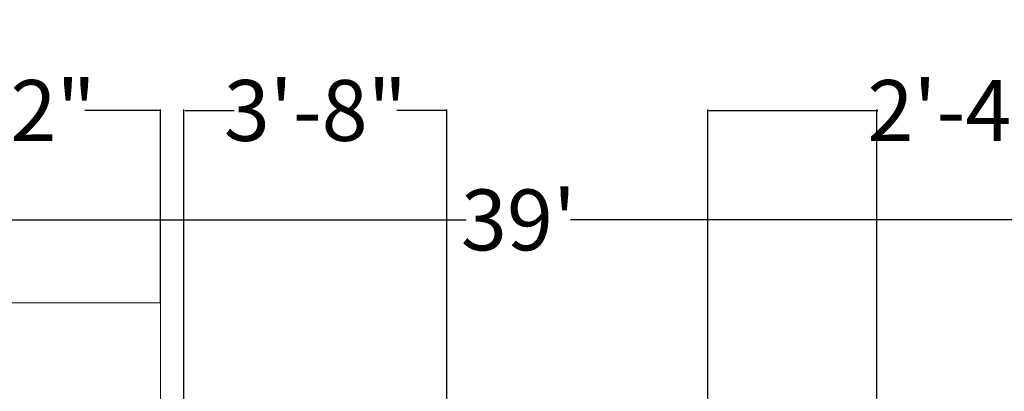
# Model space of a CAD drawing. Units: inches. Extents: x 2379 to 3013, y 1431 to 2110.
# Tile 8 of 10: x 2620 to 2785, y 2047 to 2110. Entities that reach past the tile are written whole.
import ezdxf

# ---------------------------------------------------------------- set-up
doc = ezdxf.new("R2010")
doc.units = ezdxf.units.IN
doc.layers.add('A-ANNO-DIMS', color=2, linetype='Continuous', lineweight=18)
doc.layers.add('A-FLOR-STRS', color=7, linetype='Continuous', lineweight=18)
doc.styles.get("Standard").update_dxf_attribs({"font": 'arial.ttf'})
doc.dimstyles.get("Standard").update_dxf_attribs({"dimtxt": 10.18, "dimasz": 0.18, "dimexe": 0.18, "dimexo": 0.0625, "dimgap": 0.09, "dimtad": 0, "dimtih": 1, "dimtoh": 1, "dimdec": 0, "dimzin": 0, "dimdsep": 46, "dimlunit": 3, "dimtxsty": 'Standard', "dimcen": 0.09, "dimadec": 0, "dimazin": 0, "dimtfac": 1, "dimtdec": 0, "dimtofl": 0, "dimtmove": 0, "dimatfit": 3, "dimfxl": 1, "dimtolj": 1, "dimtzin": 0, "dimarcsym": 0})

# ---------------------------------------------------------------- blocks, each defined once
blk = doc.blocks.new('*D14')
at = {"layer": 'A-ANNO-DIMS', "color": 0, "lineweight": -2, "transparency": 16777216}
for p, q in [((2469.63, 2021.67), (2469.63, 2076.34)), ((2469.81, 2076.16), (2694.9, 2076.16)), ((2937.45, 2076.16), (2712.35, 2076.16)), ((2937.63, 2021.67), (2937.63, 2076.34))]:
    blk.add_line(p, q, dxfattribs=at)
at = {"layer": 'A-ANNO-DIMS', "color": 0, "transparency": 16777216}
for points in [[(2469.81, 2076.19), (2469.81, 2076.13), (2469.63, 2076.16)], [(2937.45, 2076.19), (2937.45, 2076.13), (2937.63, 2076.16)]]:
    blk.add_solid(points, dxfattribs=at)
at = {"layer": 'Defpoints', "color": 0, "transparency": 16777216}
for p in [(2937.63, 2076.16), (2469.63, 2021.61), (2937.63, 2021.61)]:
    blk.add_point(p, dxfattribs=at)
at = {"layer": 'A-ANNO-DIMS', "color": 0, "transparency": 16777216, "insert": (2703.63, 2076.16), "char_height": 10.18, "attachment_point": 5}
blk.add_mtext("\\A1;39'", dxfattribs=at)
blk = doc.blocks.new('*D28')
at = {"layer": 'A-ANNO-DIMS', "color": 0, "lineweight": -2, "transparency": 16777216}
for p, q in [((2714.17, 2021.67), (2714.17, 2025.39)), ((2714.35, 2025.21), (2737.99, 2025.21)), ((2738.17, 2021.67), (2738.17, 2025.39)), ((2738.17, 2025.21), (2738.35, 2025.21))]:
    blk.add_line(p, q, dxfattribs=at)
at = {"layer": 'A-ANNO-DIMS', "color": 0, "transparency": 16777216}
for points in [[(2714.35, 2025.24), (2714.35, 2025.18), (2714.17, 2025.21)], [(2737.99, 2025.24), (2737.99, 2025.18), (2738.17, 2025.21)]]:
    blk.add_solid(points, dxfattribs=at)
at = {"layer": 'Defpoints', "color": 0, "transparency": 16777216}
for p in [(2738.17, 2025.21), (2714.17, 2021.61), (2738.17, 2021.61)]:
    blk.add_point(p, dxfattribs=at)
at = {"layer": 'A-ANNO-DIMS', "color": 0, "transparency": 16777216, "insert": (2797.39, 2025.21), "char_height": 10.18, "attachment_point": 5}
blk.add_mtext('\\A1;VENT V 2\'-0" TYP.', dxfattribs=at)
blk = doc.blocks.new('*D30')
at = {"layer": 'A-ANNO-DIMS', "color": 0, "lineweight": -2, "transparency": 16777216}
for p, q in [((2800.26, 2026.41), (2800.08, 2026.41)), ((2800.26, 2011.63), (2800.26, 2026.59)), ((2899.08, 2026.41), (2800.44, 2026.41)), ((2899.26, 2011.63), (2899.26, 2026.59))]:
    blk.add_line(p, q, dxfattribs=at)
at = {"layer": 'A-ANNO-DIMS', "color": 0, "transparency": 16777216}
for points in [[(2800.44, 2026.44), (2800.44, 2026.38), (2800.26, 2026.41)], [(2899.08, 2026.44), (2899.08, 2026.38), (2899.26, 2026.41)]]:
    blk.add_solid(points, dxfattribs=at)
at = {"layer": 'Defpoints', "color": 0, "transparency": 16777216}
for p in [(2800.26, 2026.41), (2800.26, 2011.56), (2899.26, 2011.56)]:
    blk.add_point(p, dxfattribs=at)
at = {"layer": 'A-ANNO-DIMS', "color": 0, "transparency": 16777216, "insert": (2724.54, 2026.41), "char_height": 10.18, "attachment_point": 5}
blk.add_mtext('\\A1;BED GROUP 8\'-3" TYP.', dxfattribs=at)
blk = doc.blocks.new('*D51')
at = {"layer": 'A-ANNO-DIMS', "color": 0, "lineweight": -2, "transparency": 16777216}
for p, q in [((2567.4, 2062.32), (2567.4, 2094.64)), ((2567.58, 2094.46), (2580.04, 2094.46)), ((2643.52, 2094.46), (2631.06, 2094.46)), ((2643.7, 2062.32), (2643.7, 2094.64))]:
    blk.add_line(p, q, dxfattribs=at)
at = {"layer": 'A-ANNO-DIMS', "color": 0, "transparency": 16777216}
for points in [[(2567.58, 2094.49), (2567.58, 2094.43), (2567.4, 2094.46)], [(2643.52, 2094.49), (2643.52, 2094.43), (2643.7, 2094.46)]]:
    blk.add_solid(points, dxfattribs=at)
at = {"layer": 'Defpoints', "color": 0, "transparency": 16777216}
for p in [(2643.7, 2094.46), (2567.4, 2062.26), (2643.7, 2062.26)]:
    blk.add_point(p, dxfattribs=at)
at = {"layer": 'A-ANNO-DIMS', "color": 0, "transparency": 16777216, "insert": (2605.55, 2094.46), "char_height": 10.18, "attachment_point": 5}
blk.add_mtext('\\A1;6\'-4 1/2"', dxfattribs=at)
blk = doc.blocks.new('*D55')
at = {"layer": 'A-ANNO-DIMS', "color": 0, "lineweight": -2, "transparency": 16777216}
for p, q in [((2647.63, 2012.67), (2647.63, 2094.64)), ((2647.81, 2094.46), (2656.01, 2094.46)), ((2691.45, 2094.46), (2683.25, 2094.46)), ((2691.63, 2012.67), (2691.63, 2094.64))]:
    blk.add_line(p, q, dxfattribs=at)
at = {"layer": 'A-ANNO-DIMS', "color": 0, "transparency": 16777216}
for points in [[(2647.81, 2094.49), (2647.81, 2094.43), (2647.63, 2094.46)], [(2691.45, 2094.49), (2691.45, 2094.43), (2691.63, 2094.46)]]:
    blk.add_solid(points, dxfattribs=at)
at = {"layer": 'Defpoints', "color": 0, "transparency": 16777216}
for p in [(2691.63, 2094.46), (2647.63, 2012.61), (2691.63, 2012.61)]:
    blk.add_point(p, dxfattribs=at)
at = {"layer": 'A-ANNO-DIMS', "color": 0, "transparency": 16777216, "insert": (2669.63, 2094.46), "char_height": 10.18, "attachment_point": 5}
blk.add_mtext('\\A1;3\'-8"', dxfattribs=at)
blk = doc.blocks.new('*D65')
at = {"layer": 'A-ANNO-DIMS', "color": 0, "lineweight": -2, "transparency": 16777216}
for p, q in [((2735.32, 1920.86), (2735.32, 2094.64)), ((2735.5, 2094.46), (2763.45, 2094.46)), ((2763.63, 1924.67), (2763.63, 2094.64)), ((2763.63, 2094.46), (2763.81, 2094.46))]:
    blk.add_line(p, q, dxfattribs=at)
at = {"layer": 'A-ANNO-DIMS', "color": 0, "transparency": 16777216}
for points in [[(2735.5, 2094.49), (2735.5, 2094.43), (2735.32, 2094.46)], [(2763.45, 2094.49), (2763.45, 2094.43), (2763.63, 2094.46)]]:
    blk.add_solid(points, dxfattribs=at)
at = {"layer": 'Defpoints', "color": 0, "transparency": 16777216}
for p in [(2763.63, 2094.46), (2763.63, 1924.61), (2735.32, 1920.79)]:
    blk.add_point(p, dxfattribs=at)
at = {"layer": 'A-ANNO-DIMS', "color": 0, "transparency": 16777216, "insert": (2789.38, 2094.46), "char_height": 10.18, "attachment_point": 5}
blk.add_mtext('\\A1;2\'-4 1/2"', dxfattribs=at)

msp = doc.modelspace()

# ---------------------------------------------------------------- linework, layer by layer
at = {"layer": 'A-FLOR-STRS'}
for p, q in [((2643.7, 2062.26), (2567.4, 2062.26)), ((2643.7, 2021.61), (2643.7, 2062.26))]:
    msp.add_line(p, q, dxfattribs=at)

# ---------------------------------------------------------------- dimensions: what is measured, and where the dimension line sits
at = {"layer": 'A-ANNO-DIMS'}
for base, p1, p2, override, picture, middle in [((2643.7, 2094.46), (2567.4, 2062.26), (2643.7, 2062.26), {"dimdec": 1, "dimlfac": 1, "dimrnd": 0, "dimzin": 1, "dimdsep": 46, "dimlunit": 4, "dimfrac": 2}, '*D51', (2605.55, 2094.46)), ((2763.63, 2094.46), (2735.32, 1920.79), (2763.63, 1924.61), {"dimdec": 1, "dimlfac": 1, "dimrnd": 0, "dimzin": 1, "dimdsep": 46, "dimlunit": 4, "dimfrac": 2}, '*D65', (2789.38, 2094.46)), ((2691.63, 2094.46), (2647.63, 2012.61), (2691.63, 2012.61), {"dimdec": 1, "dimlfac": 1, "dimrnd": 0, "dimzin": 1, "dimdsep": 46, "dimlunit": 4, "dimfrac": 2}, '*D55', (2669.63, 2094.46)), ((2937.63, 2076.16), (2469.63, 2021.61), (2937.63, 2021.61), {"dimclrd": 0, "dimclre": 0, "dimclrt": 0}, '*D14', (2703.63, 2076.16))]:
    dim = msp.add_linear_dim(base=base, p1=p1, p2=p2, dimstyle='Standard', override=override, dxfattribs=at)
    dim.commit()
    dim.dimension.update_dxf_attribs({"geometry": picture, "text_midpoint": middle})
dim = msp.add_linear_dim(base=(2800.26, 2026.41), p1=(2899.26, 2011.56), p2=(2800.26, 2011.56), angle=180, text='BED GROUP <> TYP.', dimstyle='Standard', override={"dimdec": 1, "dimlfac": 1, "dimrnd": 0, "dimzin": 1, "dimdsep": 46, "dimlunit": 4, "dimfrac": 2}, dxfattribs=at)
dim.commit()
dim.dimension.update_dxf_attribs({"geometry": '*D30', "text_midpoint": (2724.54, 2026.41)})
dim = msp.add_linear_dim(base=(2738.17, 2025.21), p1=(2714.17, 2021.61), p2=(2738.17, 2021.61), text='VENT V <> TYP.', dimstyle='Standard', override={"dimdec": 1, "dimlfac": 1, "dimrnd": 0, "dimzin": 1, "dimdsep": 46, "dimlunit": 4, "dimfrac": 2}, dxfattribs=at)
dim.commit()
dim.dimension.update_dxf_attribs({"geometry": '*D28', "text_midpoint": (2797.39, 2025.21)})

doc.saveas('drawing.dxf')
